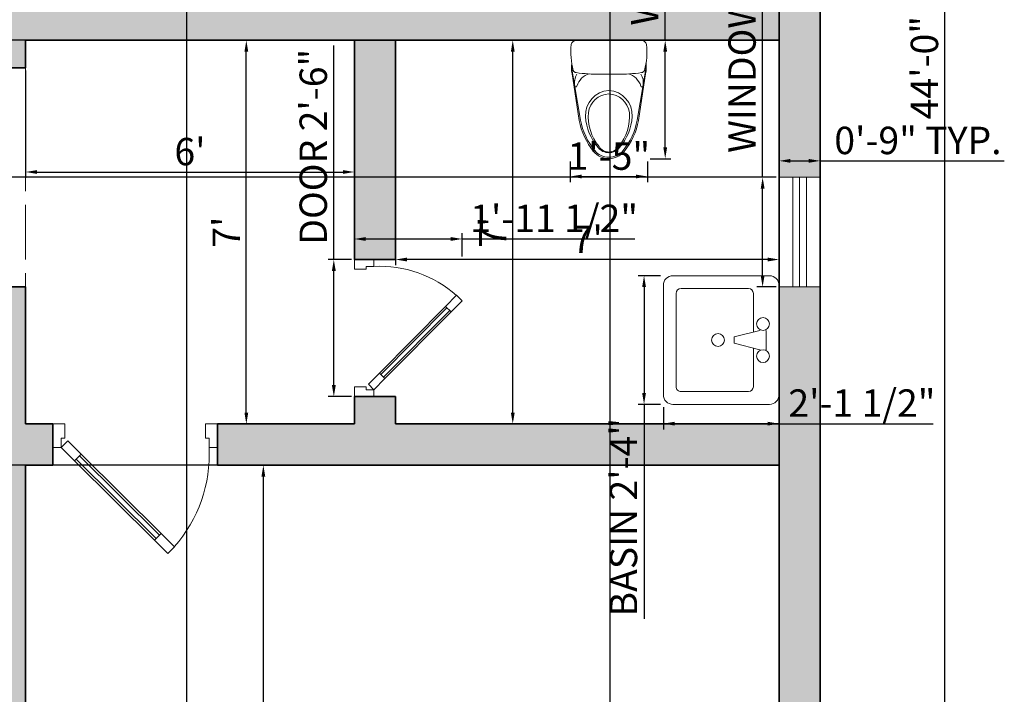
# Model space of a CAD drawing. Units: inches. Extents: x -40 to 424, y -33 to 568.
# Tile 3 of 8: x 209 to 424, y 127 to 275. Entities that reach past the tile are written whole.
import ezdxf

# ---------------------------------------------------------------- set-up
doc = ezdxf.new("R2010")
doc.units = ezdxf.units.IN
doc.linetypes.add('ACAD_ISO02W100', pattern=[15, 12, -3])
for name, color, linetype, lineweight in [('A-ANNO-DIMS', 7, 'Continuous', 18), ('A-DOOR', 7, 'Continuous', 18), ('A-FLOR-FIXT', 7, 'Continuous', 18), ('A-GLAZ', 7, 'Continuous', 18), ('A-WALL-OVHD', 7, 'ACAD_ISO02W100', 18), ('A-WALL-PATT', 30, 'Continuous', 13), ('wall', 7, 'Continuous', 35)]:
    doc.layers.add(name, color=color, linetype=linetype, lineweight=lineweight)
doc.styles.get("Standard").update_dxf_attribs({"font": 'arial.ttf'})
doc.dimstyles.new('ISO-25', dxfattribs={"dimtxt": 6, "dimasz": 2.5, "dimexe": 1.25, "dimexo": 0.625, "dimtad": 1, "dimdec": 1, "dimlunit": 3, "dimtxsty": 'Standard', "dimcen": 2.5, "dimadec": 0, "dimazin": 0, "dimtfac": 1, "dimtdec": 1, "dimtmove": 0, "dimatfit": 3, "dimfxl": 1, "dimarcsym": 0})

# ---------------------------------------------------------------- blocks, each defined once
blk = doc.blocks.new('A$C3C032968')
for p, q in [((0, 0), (0, 100)), ((0, 100), (0, 0)), ((700, 0), (700, 100)), ((700, 0), (700, 100))]:
    blk.add_line(p, q)
for points in [[(517.5, 522.4), (460.7, 466.1), (432.5, 494.5), (489.3, 550.8)], [(120, 128), (460.7, 466.1), (432.5, 494.5), (91.8, 156.4)], [(112.9, 135.1), (453.6, 473.2), (439.5, 487.4), (98.8, 149.3)], [(63.2, 71.6), (120, 128), (91.8, 156.4), (35, 100)], [(35, 100), (0, 100), (0, 0), (50, 0), (50, 50), (50, 60), (35, 60)], [(665, 100), (665, 60), (650, 60), (650, 50), (650, 0), (700, 0), (700, 100)]]:
    blk.add_lwpolyline(points, close=True)
blk.add_arc((72.4, 128.7), 593.3, 357.2313, 41.4937)
blk = doc.blocks.new('A$C329C6BD7')
at = {"linetype": 'ByBlock'}
for p, q in [((0.4699, 0.4572), (0.0381, 0.4572)), ((0, 0.4191), (0, 0.0381)), ((0.2159, 0.4064), (0.2921, 0.4064)), ((0.508, 0.0381), (0.508, 0.4191)), ((0.0698, 0.3556), (0.2223, 0.3556)), ((0.2159, 0.381), (0.2413, 0.2794)), ((0.2667, 0.2794), (0.2921, 0.381)), ((0.2858, 0.3556), (0.4382, 0.3556)), ((0.0508, 0.0698), (0.0508, 0.3365)), ((0.4572, 0.3365), (0.4572, 0.0698)), ((0.2413, 0.2794), (0.2667, 0.2794)), ((0.4382, 0.0508), (0.0698, 0.0508)), ((0.0381, 0), (0.4699, 0))]:
    blk.add_line(p, q, dxfattribs=at)
for centre in [(0.1905, 0.3937), (0.3175, 0.3937), (0.254, 0.2159)]:
    blk.add_circle(centre, 0.0254, dxfattribs=at)
for centre, radius, start, end in [((0.0381, 0.4191), 0.0381, 90, 180), ((0.4699, 0.4191), 0.0381, 0, 90), ((0.0698, 0.3365), 0.0191, 90, 180), ((0.4382, 0.3365), 0.0191, 0, 90), ((0.0698, 0.0698), 0.0191, 180, 270), ((0.4382, 0.0698), 0.0191, 270, 0), ((0.0381, 0.0381), 0.0381, 180, 270), ((0.4699, 0.0381), 0.0381, 270, 0)]:
    blk.add_arc(centre, radius, start, end, dxfattribs=at)
blk = doc.blocks.new('A$C188A4A68')
at = {"ltscale": 20}
for p, q in [((0.2444, 0.7693), (0.0344, 0.7693)), ((0.2444, 0.7693), (0.4544, 0.7693)), ((0.0013, 0.5938), (0.0607, 0.2504)), ((0.4874, 0.5938), (0.428, 0.2504)), ((0.0054, 0.5515), (0.0519, 0.2489)), ((0.2444, 0.5498), (0.1889, 0.5498)), ((0.2444, 0.5498), (0.2998, 0.5498)), ((0.4833, 0.5515), (0.4368, 0.2489))]:
    blk.add_line(p, q, dxfattribs=at)
for centre, radius, start, end in [((0.0344, 0.7343), 0.0349, 90, 169.59261), ((0.4544, 0.7343), 0.0349, 10.40739, 90), ((0.442, 0.6914), 0.4447, 173.63949, 195.46404), ((0.0467, 0.6914), 0.4447, 344.53596, 6.36051), ((0.2125, 0.5932), 0.2113, 172.64979, 191.36585), ((0.2762, 0.5932), 0.2113, 348.63415, 7.35021), ((0.0333, 0.5802), 0.0213, 200.24298, 267.15028), ((0.1303, 0.4913), 0.1097, 148.50689, 190.04883), ((0.1632, 1.4554), 0.906, 261.69023, 271.62576), ((0.1461, 0.4405), 0.1134, 104.10408, 164.15012), ((0.3255, 1.4554), 0.906, 268.37424, 278.30977), ((0.3426, 0.4405), 0.1134, 15.84988, 75.89592), ((0.3584, 0.4913), 0.1097, 349.95117, 31.49311), ((0.4554, 0.5802), 0.0213, 272.84972, 339.75702), ((0.0297, 0.4734), 0.0075, 189.82636, 345.08753), ((0.459, 0.4734), 0.0075, 194.91247, 350.17364), ((0.254, 0.2824), 0.1613, 93.43328, 183.00378), ((0.2493, 0.2813), 0.1393, 92.03292, 172.03731), ((0.2347, 0.2824), 0.1613, 356.99622, 86.56672), ((0.2394, 0.2813), 0.1393, 7.96269, 87.96708), ((0.4311, 0.2946), 0.3389, 183.50421, 221.02292), ((0.4211, 0.2752), 0.3108, 175.32131, 219.24773), ((0.0676, 0.2752), 0.3108, 320.75227, 4.67869), ((0.0576, 0.2946), 0.3389, 318.97708, 356.49579), ((0.4781, 0.3243), 0.4328, 190.02971, 219.74275), ((0.4781, 0.3243), 0.4238, 190.04347, 219.7538), ((0.0106, 0.3243), 0.4238, 320.2462, 349.95653), ((0.0106, 0.3243), 0.4328, 320.25725, 349.97029), ((0.2444, 0.127), 0.088, 218.504, 270), ((0.2498, 0.1282), 0.0854, 215.56846, 266.31968), ((0.2389, 0.1282), 0.0854, 273.68032, 324.43154), ((0.2444, 0.127), 0.088, 270, 321.496), ((0.2444, 0.127), 0.127, 218.71605, 270), ((0.2444, 0.127), 0.118, 218.67741, 270), ((0.2444, 0.127), 0.118, 270, 321.32259), ((0.2444, 0.127), 0.127, 270, 321.28395)]:
    blk.add_arc(centre, radius, start, end, dxfattribs=at)
blk = doc.blocks.new('*D20')
at = {"layer": 'A-ANNO-DIMS', "color": 0, "lineweight": -2, "transparency": 16777216}
for p, q in [((262.04, 177), (260.82, 177)), ((262.07, 11.5), (262.07, 174.5)), ((262.04, 9), (260.82, 9))]:
    blk.add_line(p, q, dxfattribs=at)
at = {"layer": 'A-ANNO-DIMS', "color": 0, "transparency": 16777216}
for points in [[(261.66, 174.5), (262.49, 174.5), (262.07, 177)], [(261.66, 11.5), (262.49, 11.5), (262.07, 9)]]:
    blk.add_solid(points, dxfattribs=at)
at = {"layer": 'Defpoints', "color": 0, "transparency": 16777216}
for p in [(262.07, 177), (262.66, 177), (262.66, 9)]:
    blk.add_point(p, dxfattribs=at)
at = {"layer": 'A-ANNO-DIMS', "color": 0, "transparency": 16777216, "insert": (258.44, 93), "char_height": 6, "attachment_point": 5, "rotation": 90}
blk.add_mtext("14'", dxfattribs=at)
blk = doc.blocks.new('*D21')
at = {"layer": 'A-ANNO-DIMS', "color": 0, "lineweight": -2, "transparency": 16777216}
for p, q in [((318.41, 270), (315.43, 270)), ((316.68, 188.5), (316.68, 267.5)), ((318.41, 186), (315.43, 186))]:
    blk.add_line(p, q, dxfattribs=at)
at = {"layer": 'A-ANNO-DIMS', "color": 0, "transparency": 16777216}
for points in [[(316.27, 267.5), (317.1, 267.5), (316.68, 270)], [(316.27, 188.5), (317.1, 188.5), (316.68, 186)]]:
    blk.add_solid(points, dxfattribs=at)
at = {"layer": 'Defpoints', "color": 0, "transparency": 16777216}
for p in [(316.68, 270), (319.03, 270), (319.03, 186)]:
    blk.add_point(p, dxfattribs=at)
at = {"layer": 'A-ANNO-DIMS', "color": 0, "transparency": 16777216, "insert": (313.06, 228), "char_height": 6, "attachment_point": 5, "rotation": 90}
blk.add_mtext("7'", dxfattribs=at)
blk = doc.blocks.new('*D22')
at = {"layer": 'A-ANNO-DIMS', "color": 0, "lineweight": -2, "transparency": 16777216}
for p, q in [((291, 252.35), (291, 220.75)), ((375, 252.35), (375, 220.75)), ((372.5, 222), (293.5, 222))]:
    blk.add_line(p, q, dxfattribs=at)
at = {"layer": 'A-ANNO-DIMS', "color": 0, "transparency": 16777216}
for points in [[(293.5, 222.42), (293.5, 221.58), (291, 222)], [(372.5, 222.42), (372.5, 221.58), (375, 222)]]:
    blk.add_solid(points, dxfattribs=at)
at = {"layer": 'Defpoints', "color": 0, "transparency": 16777216}
for p in [(291, 252.98), (375, 252.98), (291, 222)]:
    blk.add_point(p, dxfattribs=at)
at = {"layer": 'A-ANNO-DIMS', "color": 0, "transparency": 16777216, "insert": (333, 225.62), "char_height": 6, "attachment_point": 5}
blk.add_mtext("7'", dxfattribs=at)
blk = doc.blocks.new('*D25')
at = {"layer": 'A-ANNO-DIMS', "color": 0, "lineweight": -2, "transparency": 16777216}
for p, q in [((210, 263.38), (210, 239.91)), ((282, 263.38), (282, 239.91)), ((212.5, 241.16), (279.5, 241.16))]:
    blk.add_line(p, q, dxfattribs=at)
at = {"layer": 'A-ANNO-DIMS', "color": 0, "transparency": 16777216}
for points in [[(212.5, 241.58), (212.5, 240.75), (210, 241.16)], [(279.5, 241.58), (279.5, 240.75), (282, 241.16)]]:
    blk.add_solid(points, dxfattribs=at)
at = {"layer": 'Defpoints', "color": 0, "transparency": 16777216}
for p in [(210, 264), (282, 264), (282, 241.16)]:
    blk.add_point(p, dxfattribs=at)
at = {"layer": 'A-ANNO-DIMS', "color": 0, "transparency": 16777216, "insert": (246, 244.85), "char_height": 6, "attachment_point": 5}
blk.add_mtext("6'", dxfattribs=at)
blk = doc.blocks.new('*D26')
at = {"layer": 'A-ANNO-DIMS', "color": 0, "lineweight": -2, "transparency": 16777216}
for p, q in [((258.97, 270), (259.59, 270)), ((258.34, 188.5), (258.34, 267.5)), ((258.97, 186), (259.59, 186))]:
    blk.add_line(p, q, dxfattribs=at)
at = {"layer": 'A-ANNO-DIMS', "color": 0, "transparency": 16777216}
for points in [[(257.93, 267.5), (258.76, 267.5), (258.34, 270)], [(257.93, 188.5), (258.76, 188.5), (258.34, 186)]]:
    blk.add_solid(points, dxfattribs=at)
at = {"layer": 'Defpoints', "color": 0, "transparency": 16777216}
for p in [(258.34, 270), (258.34, 270), (258.34, 186)]:
    blk.add_point(p, dxfattribs=at)
at = {"layer": 'A-ANNO-DIMS', "color": 0, "transparency": 16777216, "insert": (254.72, 228), "char_height": 6, "attachment_point": 5, "rotation": 90}
blk.add_mtext("7'", dxfattribs=at)
blk = doc.blocks.new('WIN-24IN')
for p, q in [((9, 24), (0, 24)), ((3, 0), (3, 24)), ((4.5, 0), (4.5, 24)), ((6, 0), (6, 24)), ((9, 0), (0, 0))]:
    blk.add_line(p, q)
blk = doc.blocks.new('*D45')
at = {"layer": 'A-ANNO-DIMS', "color": 0, "lineweight": -2, "transparency": 16777216}
for p, q in [((371.4, 240), (371.4, 334.58)), ((374.38, 240), (370.15, 240)), ((371.4, 218.5), (371.4, 237.5)), ((374.38, 216), (370.15, 216))]:
    blk.add_line(p, q, dxfattribs=at)
at = {"layer": 'A-ANNO-DIMS', "color": 0, "transparency": 16777216}
for points in [[(370.98, 237.5), (371.82, 237.5), (371.4, 240)], [(370.98, 218.5), (371.82, 218.5), (371.4, 216)]]:
    blk.add_solid(points, dxfattribs=at)
at = {"layer": 'Defpoints', "color": 0, "transparency": 16777216}
for p in [(371.4, 240), (375, 240), (375, 216)]:
    blk.add_point(p, dxfattribs=at)
at = {"layer": 'A-ANNO-DIMS', "color": 0, "transparency": 16777216, "insert": (367.67, 288.54), "char_height": 6, "attachment_point": 5, "rotation": 90}
blk.add_mtext('WINDOW W2 2\'-0" TYP.', dxfattribs=at)
blk = doc.blocks.new('*D46')
at = {"layer": 'A-ANNO-DIMS', "color": 0, "lineweight": -2, "transparency": 16777216}
for p, q in [((375, 240.62), (375, 244.85)), ((384, 240.62), (384, 244.85)), ((377.5, 243.6), (381.5, 243.6)), ((384, 243.6), (424.32, 243.6))]:
    blk.add_line(p, q, dxfattribs=at)
at = {"layer": 'A-ANNO-DIMS', "color": 0, "transparency": 16777216}
for points in [[(377.5, 244.02), (377.5, 243.18), (375, 243.6)], [(381.5, 244.02), (381.5, 243.18), (384, 243.6)]]:
    blk.add_solid(points, dxfattribs=at)
at = {"layer": 'Defpoints', "color": 0, "transparency": 16777216}
for p in [(384, 243.6), (375, 240), (384, 240)]:
    blk.add_point(p, dxfattribs=at)
at = {"layer": 'A-ANNO-DIMS', "color": 0, "transparency": 16777216, "insert": (405.41, 247.29), "char_height": 6, "attachment_point": 5}
blk.add_mtext('0\'-9" TYP.', dxfattribs=at)
blk = doc.blocks.new('*D49')
at = {"layer": 'A-ANNO-DIMS', "color": 0, "lineweight": -2, "transparency": 16777216}
for p, q in [((277.5, 222), (277.5, 268.88)), ((281.38, 222), (276.25, 222)), ((277.5, 194.5), (277.5, 219.5)), ((281.38, 192), (276.25, 192))]:
    blk.add_line(p, q, dxfattribs=at)
at = {"layer": 'A-ANNO-DIMS', "color": 0, "transparency": 16777216}
for points in [[(277.08, 219.5), (277.92, 219.5), (277.5, 222)], [(277.08, 194.5), (277.92, 194.5), (277.5, 192)]]:
    blk.add_solid(points, dxfattribs=at)
at = {"layer": 'Defpoints', "color": 0, "transparency": 16777216}
for p in [(277.5, 222), (282, 222), (282, 192)]:
    blk.add_point(p, dxfattribs=at)
at = {"layer": 'A-ANNO-DIMS', "color": 0, "transparency": 16777216, "insert": (273.77, 246.69), "char_height": 6, "attachment_point": 5, "rotation": 90}
blk.add_mtext('DOOR 2\'-6"', dxfattribs=at)
blk = doc.blocks.new('*D50')
at = {"layer": 'A-ANNO-DIMS', "color": 0, "lineweight": -2, "transparency": 16777216}
for p, q in [((282, 222.63), (282, 227.75)), ((284.5, 226.5), (303.11, 226.5)), ((305.61, 222.63), (305.61, 227.75)), ((305.61, 226.5), (343.38, 226.5))]:
    blk.add_line(p, q, dxfattribs=at)
at = {"layer": 'A-ANNO-DIMS', "color": 0, "transparency": 16777216}
for points in [[(284.5, 226.92), (284.5, 226.08), (282, 226.5)], [(303.11, 226.92), (303.11, 226.08), (305.61, 226.5)]]:
    blk.add_solid(points, dxfattribs=at)
at = {"layer": 'Defpoints', "color": 0, "transparency": 16777216}
for p in [(305.61, 226.5), (282, 222), (305.61, 222)]:
    blk.add_point(p, dxfattribs=at)
at = {"layer": 'A-ANNO-DIMS', "color": 0, "transparency": 16777216, "insert": (325.74, 230.23), "char_height": 6, "attachment_point": 5}
blk.add_mtext('1\'-11 1/2"', dxfattribs=at)
blk = doc.blocks.new('*D65')
at = {"layer": 'A-ANNO-DIMS', "color": 0, "lineweight": -2, "transparency": 16777216}
for p, q in [((349.03, 218.46), (344.18, 218.46)), ((345.43, 215.96), (345.43, 192.8)), ((349.03, 190.3), (344.18, 190.3)), ((345.43, 190.3), (345.43, 143.38))]:
    blk.add_line(p, q, dxfattribs=at)
at = {"layer": 'A-ANNO-DIMS', "color": 0, "transparency": 16777216}
for points in [[(345.02, 215.96), (345.85, 215.96), (345.43, 218.46)], [(345.02, 192.8), (345.85, 192.8), (345.43, 190.3)]]:
    blk.add_solid(points, dxfattribs=at)
at = {"layer": 'Defpoints', "color": 0, "transparency": 16777216}
for p in [(349.66, 218.46), (345.43, 190.3), (349.66, 190.3)]:
    blk.add_point(p, dxfattribs=at)
at = {"layer": 'A-ANNO-DIMS', "color": 0, "transparency": 16777216, "insert": (341.7, 165.59), "char_height": 6, "attachment_point": 5, "rotation": 90}
blk.add_mtext('BASIN 2\'-4"', dxfattribs=at)
blk = doc.blocks.new('*D66')
at = {"layer": 'A-ANNO-DIMS', "color": 0, "lineweight": -2, "transparency": 16777216}
for p, q in [((349.66, 189.67), (349.66, 184.82)), ((375, 189.67), (375, 184.82)), ((352.16, 186.07), (372.5, 186.07)), ((375, 186.07), (408.78, 186.07))]:
    blk.add_line(p, q, dxfattribs=at)
at = {"layer": 'A-ANNO-DIMS', "color": 0, "transparency": 16777216}
for points in [[(352.16, 186.49), (352.16, 185.66), (349.66, 186.07)], [(372.5, 186.49), (372.5, 185.66), (375, 186.07)]]:
    blk.add_solid(points, dxfattribs=at)
at = {"layer": 'Defpoints', "color": 0, "transparency": 16777216}
for p in [(349.66, 190.3), (375, 190.3), (375, 186.07)]:
    blk.add_point(p, dxfattribs=at)
at = {"layer": 'A-ANNO-DIMS', "color": 0, "transparency": 16777216, "insert": (393.14, 189.8), "char_height": 6, "attachment_point": 5}
blk.add_mtext('2\'-1 1/2"', dxfattribs=at)
blk = doc.blocks.new('*D69')
at = {"layer": 'A-ANNO-DIMS', "color": 0, "lineweight": -2, "transparency": 16777216}
for p, q in [((350.07, 270), (350.07, 306.24)), ((346.8, 270), (351.32, 270)), ((350.07, 246.57), (350.07, 267.5)), ((346.8, 244.07), (351.32, 244.07))]:
    blk.add_line(p, q, dxfattribs=at)
at = {"layer": 'A-ANNO-DIMS', "color": 0, "transparency": 16777216}
for points in [[(349.65, 267.5), (350.48, 267.5), (350.07, 270)], [(349.65, 246.57), (350.48, 246.57), (350.07, 244.07)]]:
    blk.add_solid(points, dxfattribs=at)
at = {"layer": 'Defpoints', "color": 0, "transparency": 16777216}
for p in [(346.18, 270), (350.07, 270), (346.18, 244.07)]:
    blk.add_point(p, dxfattribs=at)
at = {"layer": 'A-ANNO-DIMS', "color": 0, "transparency": 16777216, "insert": (346.34, 289.37), "char_height": 6, "attachment_point": 5, "rotation": 90}
blk.add_mtext('WC 2\'-2"', dxfattribs=at)
blk = doc.blocks.new('*D70')
at = {"layer": 'A-ANNO-DIMS', "color": 0, "lineweight": -2, "transparency": 16777216}
for p, q in [((329.28, 243.44), (329.28, 238.93)), ((346.18, 243.44), (346.18, 238.93)), ((331.78, 240.18), (343.68, 240.18))]:
    blk.add_line(p, q, dxfattribs=at)
at = {"layer": 'A-ANNO-DIMS', "color": 0, "transparency": 16777216}
for points in [[(331.78, 240.59), (331.78, 239.76), (329.28, 240.18)], [(343.68, 240.59), (343.68, 239.76), (346.18, 240.18)]]:
    blk.add_solid(points, dxfattribs=at)
at = {"layer": 'Defpoints', "color": 0, "transparency": 16777216}
for p in [(329.28, 244.07), (346.18, 244.07), (346.18, 240.18)]:
    blk.add_point(p, dxfattribs=at)
at = {"layer": 'A-ANNO-DIMS', "color": 0, "transparency": 16777216, "insert": (337.73, 243.86), "char_height": 6, "attachment_point": 5}
blk.add_mtext('1\'-5"', dxfattribs=at)
blk = doc.blocks.new('*D80')
at = {"layer": 'A-ANNO-DIMS', "color": 0, "lineweight": -2, "transparency": 16777216}
for p, q in [((384.63, 528), (412.55, 528)), ((411.3, 2.5), (411.3, 525.5)), ((384.63, 0), (412.55, 0))]:
    blk.add_line(p, q, dxfattribs=at)
at = {"layer": 'A-ANNO-DIMS', "color": 0, "transparency": 16777216}
for points in [[(410.88, 525.5), (411.72, 525.5), (411.3, 528)], [(410.88, 2.5), (411.72, 2.5), (411.3, 0)]]:
    blk.add_solid(points, dxfattribs=at)
at = {"layer": 'Defpoints', "color": 0, "transparency": 16777216}
for p in [(384, 528), (411.3, 528), (384, 0)]:
    blk.add_point(p, dxfattribs=at)
at = {"layer": 'A-ANNO-DIMS', "color": 0, "transparency": 16777216, "insert": (407.61, 264), "char_height": 6, "attachment_point": 5, "rotation": 90}
blk.add_mtext('44\'-0"', dxfattribs=at)
blk = doc.blocks.new('*D87')
at = {"layer": 'A-ANNO-DIMS', "color": 0, "lineweight": -2, "transparency": 16777216}
for p, q in [((374.38, 177), (-28.55, 177)), ((-27.3, 119.5), (-27.3, 174.5)), ((374.38, 117), (-28.55, 117))]:
    blk.add_line(p, q, dxfattribs=at)
at = {"layer": 'A-ANNO-DIMS', "color": 0, "transparency": 16777216}
for points in [[(-27.72, 174.5), (-26.88, 174.5), (-27.3, 177)], [(-27.72, 119.5), (-26.88, 119.5), (-27.3, 117)]]:
    blk.add_solid(points, dxfattribs=at)
at = {"layer": 'Defpoints', "color": 0, "transparency": 16777216}
for p in [(-27.3, 177), (375, 177), (375, 117)]:
    blk.add_point(p, dxfattribs=at)
at = {"layer": 'A-ANNO-DIMS', "color": 0, "transparency": 16777216, "insert": (-30.99, 147), "char_height": 6, "attachment_point": 5, "rotation": 90}
blk.add_mtext('5\'-0"', dxfattribs=at)
blk = doc.blocks.new('*D88')
at = {"layer": 'A-ANNO-DIMS', "color": 0, "lineweight": -2, "transparency": 16777216}
for p, q in [((374.38, 270), (-28.55, 270)), ((-27.3, 242.5), (-27.3, 267.5)), ((374.38, 240), (-28.55, 240))]:
    blk.add_line(p, q, dxfattribs=at)
at = {"layer": 'A-ANNO-DIMS', "color": 0, "transparency": 16777216}
for points in [[(-27.72, 267.5), (-26.88, 267.5), (-27.3, 270)], [(-27.72, 242.5), (-26.88, 242.5), (-27.3, 240)]]:
    blk.add_solid(points, dxfattribs=at)
at = {"layer": 'Defpoints', "color": 0, "transparency": 16777216}
for p in [(-27.3, 270), (375, 270), (375, 240)]:
    blk.add_point(p, dxfattribs=at)
at = {"layer": 'A-ANNO-DIMS', "color": 0, "transparency": 16777216, "insert": (-30.99, 255), "char_height": 6, "attachment_point": 5, "rotation": 90}
blk.add_mtext('2\'-6"', dxfattribs=at)
blk = doc.blocks.new('*D95')
at = {"layer": 'A-ANNO-DIMS', "color": 0, "lineweight": -2, "transparency": 16777216}
for p, q in [((375, 333.88), (375, -28.55)), ((337.92, 320.88), (337.92, -28.55)), ((340.42, -27.3), (372.5, -27.3))]:
    blk.add_line(p, q, dxfattribs=at)
at = {"layer": 'A-ANNO-DIMS', "color": 0, "transparency": 16777216}
for points in [[(340.42, -26.88), (340.42, -27.72), (337.92, -27.3)], [(372.5, -26.88), (372.5, -27.72), (375, -27.3)]]:
    blk.add_solid(points, dxfattribs=at)
at = {"layer": 'Defpoints', "color": 0, "transparency": 16777216}
for p in [(375, 334.5), (337.92, 321.5), (375, -27.3)]:
    blk.add_point(p, dxfattribs=at)
at = {"layer": 'A-ANNO-DIMS', "color": 0, "transparency": 16777216, "insert": (356.46, -23.61), "char_height": 6, "attachment_point": 5}
blk.add_mtext('3\'-1"', dxfattribs=at)
blk = doc.blocks.new('*D96')
at = {"layer": 'A-ANNO-DIMS', "color": 0, "lineweight": -2, "transparency": 16777216}
for p, q in [((245.23, 320.88), (245.23, -28.55)), ((337.92, 320.88), (337.92, -28.55)), ((247.73, -27.3), (335.42, -27.3))]:
    blk.add_line(p, q, dxfattribs=at)
at = {"layer": 'A-ANNO-DIMS', "color": 0, "transparency": 16777216}
for points in [[(247.73, -26.88), (247.73, -27.72), (245.23, -27.3)], [(335.42, -26.88), (335.42, -27.72), (337.92, -27.3)]]:
    blk.add_solid(points, dxfattribs=at)
at = {"layer": 'Defpoints', "color": 0, "transparency": 16777216}
for p in [(245.23, 321.5), (337.92, 321.5), (337.92, -27.3)]:
    blk.add_point(p, dxfattribs=at)
at = {"layer": 'A-ANNO-DIMS', "color": 0, "transparency": 16777216, "insert": (291.58, -23.57), "char_height": 6, "attachment_point": 5}
blk.add_mtext('7\'-8 1/2"', dxfattribs=at)

msp = doc.modelspace()

# ---------------------------------------------------------------- hatches: boundary and pattern name
at = {"layer": 'A-WALL-PATT'}
h = msp.add_hatch(color=256, dxfattribs=at)
h.dxf.hatch_style = 1
h.paths.add_polyline_path([(9, 399), (0, 399), (0, 351), (9, 351)])
h.paths.add_polyline_path([(9, 303), (0, 303), (0, 210), (9, 210)])
h.paths.add_polyline_path([(9, 150), (0, 150), (0, 0), (384, 0), (384, 69), (375, 69), (375, 62.24), (375, 9), (9, 9)])
h.paths.add_polyline_path([(210, 177), (216, 177), (216, 186), (210, 186), (210, 216), (201, 216), (201, 90), (195, 90), (195, 81), (201, 81), (201, 9), (210, 9)])
h.paths.add_polyline_path([(384, 216), (375, 216), (375, 117), (384, 117)])
h.paths.add_polyline_path([(384, 298.5), (375, 298.5), (375, 279), (375, 240), (384, 240)])
h.paths.add_polyline_path([(384, 417), (375, 417), (375, 334.5), (384, 334.5)])
h.paths.add_polyline_path([(384, 528), (216, 528), (216, 519), (375, 519), (375, 465), (384, 465)])
h.paths.add_polyline_path([(192, 528), (0, 528), (0, 511.5), (9, 511.5), (9, 519), (192, 519)])
h.paths.add_polyline_path([(9, 487.5), (0, 487.5), (0, 447), (9, 447)])
h.paths.add_polyline_path([(111, 480), (9, 480), (9, 471), (111, 471)])
h.paths.add_polyline_path([(174, 519), (165, 519), (165, 354), (174, 354)])
h.paths.add_polyline_path([(243, 426), (237.86, 426), (234, 426), (234, 420), (174, 420), (174, 411), (234, 411), (234, 405), (239.14, 405), (243, 405)])
h.paths.add_polyline_path([(243, 519), (234, 519), (234, 460.14, -0.031638), (237.86, 460.2), (237.86, 462), (243, 462)])
h.paths.add_polyline_path([(243, 369), (234, 369), (234, 354), (375, 354), (375, 363), (243, 363)])
h.paths.add_polyline_path([(375, 279), (195, 279), (195, 270), (201, 270), (201, 264), (210, 264), (210, 270), (375, 270)])
h.paths.add_polyline_path([(291, 270), (282, 270), (282, 222), (286.29, 222), (291, 222)])
h.paths.add_polyline_path([(375, 186), (291, 186), (291, 192), (282, 192), (282, 186), (252, 186), (252, 180.86), (252, 177), (375, 177)])
h.paths.add_polyline_path([(147, 279), (9, 279), (9, 270), (147, 270)])

# ---------------------------------------------------------------- linework, layer by layer
at = {"layer": 'A-WALL-OVHD'}
msp.add_line((210, 264), (210, 216), dxfattribs=at)
at = {"layer": 'wall'}
for p, q in [((375, 9), (375, 519)), ((210, 270), (210, 264)), ((210, 270), (375, 270)), ((282, 222), (282, 270)), ((291, 222), (291, 270)), ((201, 264), (210, 264)), ((282, 222), (291, 222)), ((201, 216), (210, 216)), ((210, 216), (210, 186)), ((282, 186), (282, 192)), ((282, 192), (291, 192)), ((291, 186), (291, 192)), ((210, 186), (216, 186)), ((216, 186), (216, 177)), ((252, 186), (252, 177)), ((252, 186), (282, 186)), ((291, 186), (375, 186)), ((210, 177), (216, 177)), ((210, 177), (210, 9)), ((252, 177), (375, 177))]:
    msp.add_line(p, q, dxfattribs=at)
msp.add_lwpolyline([(0, 0), (384, 0), (384, 528), (0, 528)], close=True, dxfattribs=at)

# ---------------------------------------------------------------- block references
at = {"layer": 'A-DOOR'}
for p, xscale, yscale, zscale, rotation in [((282, 192), -0.0428571428571429, 0.0428571428571429, 0.0428571428571429, 270), ((216, 186), -0.0514285714285714, 0.0514285714285714, 0.0514285714285714, 180)]:
    msp.add_blockref('A$C3C032968', p, dxfattribs=dict(at, xscale=xscale, yscale=yscale, zscale=zscale, rotation=rotation))
at = {"layer": 'A-FLOR-FIXT', "xscale": 33.71396072414388, "yscale": 33.71396072414388, "zscale": 33.71396072414388}
msp.add_blockref('A$C188A4A68', (329.49, 244.07), dxfattribs=at)
at = {"layer": 'A-FLOR-FIXT', "xscale": 55.4333994836993, "yscale": 55.4333994836993, "zscale": 55.4333994836993, "rotation": 270}
msp.add_blockref('A$C329C6BD7', (349.66, 218.46), dxfattribs=at)
at = {"layer": 'A-GLAZ'}
msp.add_blockref('WIN-24IN', (375, 216), dxfattribs=at)

# ---------------------------------------------------------------- dimensions: what is measured, and where the dimension line sits
at = {"layer": 'A-ANNO-DIMS'}
for base, p1, p2, override, picture, middle in [((411.3, 528), (384, 0), (384, 528), {"dimdec": 1, "dimlfac": 1, "dimrnd": 0, "dimzin": 1, "dimdsep": 46, "dimlunit": 4, "dimfrac": 2}, '*D80', (407.61, 264)), ((-27.3, 270), (375, 240), (375, 270), {"dimdec": 1, "dimlfac": 1, "dimrnd": 0, "dimzin": 1, "dimdsep": 46, "dimlunit": 4, "dimfrac": 2}, '*D88', (-30.99, 255)), ((258.34, 270), (258.34, 186), (258.34, 270), {"dimclrd": 0, "dimclre": 0, "dimclrt": 0}, '*D26', (254.72, 228)), ((316.68, 270), (319.03, 186), (319.03, 270), {"dimclrd": 0, "dimclre": 0, "dimclrt": 0}, '*D21', (313.06, 228)), ((-27.3, 177), (375, 117), (375, 177), {"dimdec": 1, "dimlfac": 1, "dimrnd": 0, "dimzin": 1, "dimdsep": 46, "dimlunit": 4, "dimfrac": 2}, '*D87', (-30.99, 147)), ((262.07, 177), (262.66, 9), (262.66, 177), {"dimclrd": 0, "dimclre": 0, "dimclrt": 0}, '*D20', (258.44, 93))]:
    dim = msp.add_linear_dim(base=base, p1=p1, p2=p2, angle=90, dimstyle='ISO-25', override=override, dxfattribs=at)
    dim.commit()
    dim.dimension.update_dxf_attribs({"geometry": picture, "text_midpoint": middle})
for base, p1, p2, override, picture, middle in [((375, -27.3), (337.92, 321.5), (375, 334.5), {"dimdec": 1, "dimlfac": 1, "dimrnd": 0, "dimzin": 1, "dimdsep": 46, "dimlunit": 4, "dimfrac": 2}, '*D95', (356.46, -23.61)), ((337.92, -27.3), (245.23, 321.5), (337.92, 321.5), {"dimdec": 1, "dimlfac": 1, "dimrnd": 0, "dimzin": 1, "dimdsep": 46, "dimlunit": 4, "dimfrac": 2}, '*D96', (291.58, -23.57)), ((282, 241.16), (210, 264), (282, 264), {"dimclrd": 0, "dimclre": 0, "dimclrt": 0}, '*D25', (246, 244.85)), ((291, 222), (375, 252.98), (291, 252.98), {"dimclrd": 0, "dimclre": 0, "dimclrt": 0}, '*D22', (333, 225.62)), ((346.18, 240.18), (329.28, 244.07), (346.18, 244.07), {"dimdec": 1, "dimlfac": 1, "dimrnd": 0, "dimzin": 1, "dimdsep": 46, "dimlunit": 4, "dimfrac": 2}, '*D70', (337.73, 243.86)), ((305.61, 226.5), (282, 222), (305.61, 222), {"dimdec": 1, "dimlfac": 1, "dimrnd": 0, "dimzin": 1, "dimdsep": 46, "dimlunit": 4, "dimfrac": 2}, '*D50', (325.74, 230.23)), ((375, 186.07), (349.66, 190.3), (375, 190.3), {"dimdec": 1, "dimlfac": 1, "dimrnd": 0, "dimzin": 1, "dimdsep": 46, "dimlunit": 4, "dimfrac": 2}, '*D66', (393.14, 189.8))]:
    dim = msp.add_linear_dim(base=base, p1=p1, p2=p2, dimstyle='ISO-25', override=override, dxfattribs=at)
    dim.commit()
    dim.dimension.update_dxf_attribs({"geometry": picture, "text_midpoint": middle})
for base, p1, p2, angle, text, picture, middle in [((371.4, 240), (375, 216), (375, 240), 90, 'WINDOW W2 <> TYP.', '*D45', (367.67, 288.54)), ((350.07, 270), (346.18, 244.07), (346.18, 270), 90, 'WC <>', '*D69', (346.34, 289.37)), ((277.5, 222), (282, 192), (282, 222), 90, 'DOOR <>', '*D49', (273.77, 246.69)), ((345.43, 190.3), (349.66, 218.46), (349.66, 190.3), 270, 'BASIN <>', '*D65', (341.7, 165.59))]:
    dim = msp.add_linear_dim(base=base, p1=p1, p2=p2, angle=angle, text=text, dimstyle='ISO-25', override={"dimdec": 1, "dimlfac": 1, "dimrnd": 0, "dimzin": 1, "dimdsep": 46, "dimlunit": 4, "dimfrac": 2}, dxfattribs=at)
    dim.commit()
    dim.dimension.update_dxf_attribs({"geometry": picture, "text_midpoint": middle})
dim = msp.add_linear_dim(base=(384, 243.6), p1=(375, 240), p2=(384, 240), text='<> TYP.', dimstyle='ISO-25', override={"dimdec": 1, "dimlfac": 1, "dimrnd": 0, "dimzin": 1, "dimdsep": 46, "dimlunit": 4, "dimfrac": 2}, dxfattribs=at)
dim.commit()
dim.dimension.update_dxf_attribs({"geometry": '*D46', "text_midpoint": (405.41, 247.29)})

doc.saveas('drawing.dxf')
